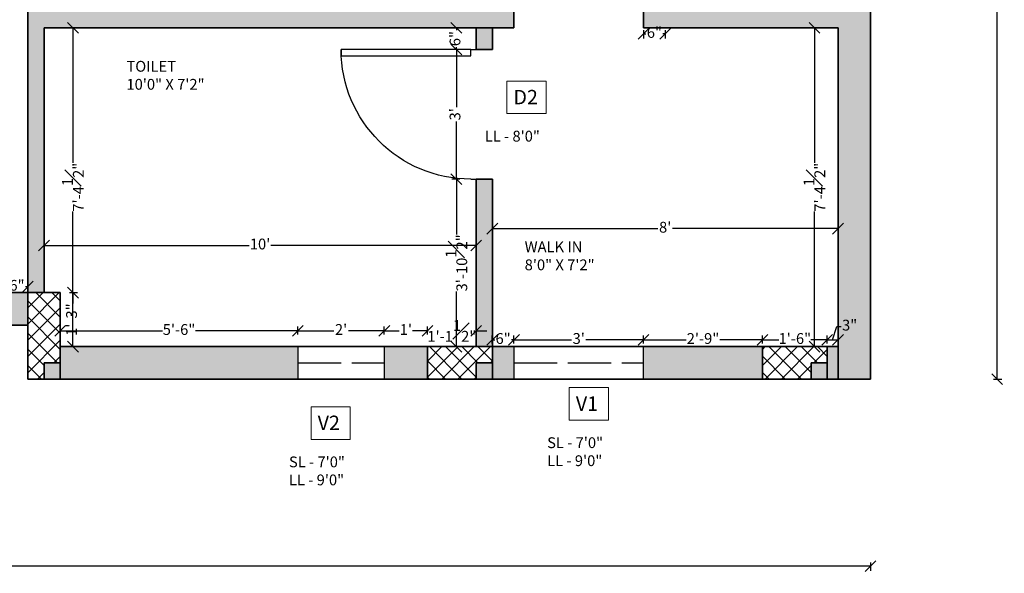
# Model space of a CAD drawing. Units: inches. Extents: x 1365 to 2091, y 1589 to 2091.
# Tile 6 of 8: x 1818 to 2091, y 1589 to 1743. Entities that reach past the tile are written whole.
import ezdxf

# ---------------------------------------------------------------- set-up
doc = ezdxf.new("R2010")
doc.units = ezdxf.units.IN
doc.linetypes.add('ACAD_ISO02W100', pattern=[15, 12, -3])
for name, color, linetype, lineweight in [('A-ANNO-DIMS', 2, 'Continuous', 18), ('A-ANNO-SYMB', 12, 'Continuous', 18), ('A-AREA-IDEN', 7, 'Continuous', 18), ('A-COLS', 7, 'Continuous', 35), ('A-COLS-MARK-PATT', 114, 'Continuous', 13), ('A-COLS-PATT', 1, 'Continuous', 13), ('A-DOOR', 4, 'Continuous', 25), ('A-GLAZ', 150, 'Continuous', 30), ('A-GLAZ-HIDN', 150, 'ACAD_ISO02W100', 30), ('A-WALL', 7, 'Continuous', 35), ('A-WALL-PATT', 253, 'Continuous', 13)]:
    doc.layers.add(name, color=color, linetype=linetype, lineweight=lineweight)
doc.styles.get("Standard").update_dxf_attribs({"font": 'arial.ttf'})
doc.dimstyles.new('ISO-25', dxfattribs={"dimtxt": 3, "dimasz": 3, "dimexe": 1.25, "dimexo": 0.625, "dimtad": 0, "dimlunit": 4, "dimtxsty": 'Standard', "dimblk": 'OBLIQUE', "dimcen": 2.5, "dimclrd": 254, "dimclre": 254, "dimclrt": 1, "dimadec": 0, "dimazin": 0, "dimtfac": 1, "dimtmove": 0, "dimatfit": 3, "dimfxl": 1, "dimfxlon": 1, "dimfrac": 1, "dimarcsym": 0})

# ---------------------------------------------------------------- blocks, each defined once
blk = doc.blocks.new('*U7')
for p, q in [((0, 0), (0, -6)), ((36, 0), (36, -6))]:
    blk.add_line(p, q)
blk.add_lwpolyline([(0, 0), (0, 36), (1.75, 36), (1.75, 0)], close=True)
blk.add_arc((0, 0), 36, 0, 90)
blk = doc.blocks.new('_Oblique')
at = {"color": 0, "linetype": 'ByBlock', "lineweight": -2}
blk.add_line((-0.5, -0.5), (0.5, 0.5), dxfattribs=at)
blk = doc.blocks.new('*D53')
at = {"layer": 'A-ANNO-DIMS', "color": 0, "lineweight": -2, "transparency": 16777216}
for p, q in [((1813.75, 1667.5), (1813.75, 1669.75)), ((1813.75, 1668.5), (1814.4, 1668.5)), ((1819.75, 1668.5), (1819.11, 1668.5)), ((1819.75, 1667.5), (1819.75, 1669.75))]:
    blk.add_line(p, q, dxfattribs=at)
at = {"layer": 'Defpoints', "color": 0, "transparency": 16777216}
for p in [(1819.75, 1668.5), (1813.75, 1666.86), (1819.75, 1666.86)]:
    blk.add_point(p, dxfattribs=at)
at = {"layer": 'A-ANNO-DIMS', "color": 0, "lineweight": -2, "transparency": 16777216, "xscale": 3, "yscale": 3, "zscale": 3, "rotation": 180}
blk.add_blockref('_Oblique', (1813.75, 1668.5), dxfattribs=at)
at = {"layer": 'A-ANNO-DIMS', "color": 0, "lineweight": -2, "transparency": 16777216, "xscale": 3, "yscale": 3, "zscale": 3}
blk.add_blockref('_Oblique', (1819.75, 1668.5), dxfattribs=at)
at = {"layer": 'A-ANNO-DIMS', "color": 0, "transparency": 16777216, "insert": (1816.75, 1668.5), "char_height": 3, "attachment_point": 5}
blk.add_mtext('6"', dxfattribs=at)
blk = doc.blocks.new('*D54')
at = {"layer": 'A-ANNO-DIMS', "color": 0, "lineweight": -2, "transparency": 16777216}
for p, q in [((1828.75, 1655.23), (1828.75, 1657.48)), ((1894.75, 1655.23), (1894.75, 1657.48)), ((1828.75, 1656.23), (1857.14, 1656.23)), ((1894.75, 1656.23), (1866.37, 1656.23))]:
    blk.add_line(p, q, dxfattribs=at)
at = {"layer": 'Defpoints', "color": 0, "transparency": 16777216}
for p in [(1894.75, 1656.23), (1828.75, 1651.86), (1894.75, 1651.86)]:
    blk.add_point(p, dxfattribs=at)
at = {"layer": 'A-ANNO-DIMS', "color": 0, "lineweight": -2, "transparency": 16777216, "xscale": 3, "yscale": 3, "zscale": 3, "rotation": 180}
blk.add_blockref('_Oblique', (1828.75, 1656.23), dxfattribs=at)
at = {"layer": 'A-ANNO-DIMS', "color": 0, "lineweight": -2, "transparency": 16777216, "xscale": 3, "yscale": 3, "zscale": 3}
blk.add_blockref('_Oblique', (1894.75, 1656.23), dxfattribs=at)
at = {"layer": 'A-ANNO-DIMS', "color": 0, "transparency": 16777216, "insert": (1861.75, 1656.23), "char_height": 3, "attachment_point": 5}
blk.add_mtext('5\'-6"', dxfattribs=at)
blk = doc.blocks.new('*D55')
at = {"layer": 'A-ANNO-DIMS', "color": 0, "lineweight": -2, "transparency": 16777216}
for p, q in [((1894.75, 1655.23), (1894.75, 1657.48)), ((1918.75, 1655.23), (1918.75, 1657.48)), ((1894.75, 1656.23), (1904.72, 1656.23)), ((1918.75, 1656.23), (1908.78, 1656.23))]:
    blk.add_line(p, q, dxfattribs=at)
at = {"layer": 'Defpoints', "color": 0, "transparency": 16777216}
for p in [(1918.75, 1656.23), (1894.75, 1651.86), (1918.75, 1651.86)]:
    blk.add_point(p, dxfattribs=at)
at = {"layer": 'A-ANNO-DIMS', "color": 0, "lineweight": -2, "transparency": 16777216, "xscale": 3, "yscale": 3, "zscale": 3, "rotation": 180}
blk.add_blockref('_Oblique', (1894.75, 1656.23), dxfattribs=at)
at = {"layer": 'A-ANNO-DIMS', "color": 0, "lineweight": -2, "transparency": 16777216, "xscale": 3, "yscale": 3, "zscale": 3}
blk.add_blockref('_Oblique', (1918.75, 1656.23), dxfattribs=at)
at = {"layer": 'A-ANNO-DIMS', "color": 0, "transparency": 16777216, "insert": (1906.75, 1656.23), "char_height": 3, "attachment_point": 5}
blk.add_mtext("2'", dxfattribs=at)
blk = doc.blocks.new('*D56')
at = {"layer": 'A-ANNO-DIMS', "color": 0, "lineweight": -2, "transparency": 16777216}
for p, q in [((1918.75, 1655.23), (1918.75, 1657.48)), ((1930.75, 1655.23), (1930.75, 1657.48)), ((1918.75, 1656.23), (1922.89, 1656.23)), ((1930.75, 1656.23), (1926.62, 1656.23))]:
    blk.add_line(p, q, dxfattribs=at)
at = {"layer": 'Defpoints', "color": 0, "transparency": 16777216}
for p in [(1930.75, 1656.23), (1918.75, 1651.86), (1930.75, 1651.86)]:
    blk.add_point(p, dxfattribs=at)
at = {"layer": 'A-ANNO-DIMS', "color": 0, "lineweight": -2, "transparency": 16777216, "xscale": 3, "yscale": 3, "zscale": 3, "rotation": 180}
blk.add_blockref('_Oblique', (1918.75, 1656.23), dxfattribs=at)
at = {"layer": 'A-ANNO-DIMS', "color": 0, "lineweight": -2, "transparency": 16777216, "xscale": 3, "yscale": 3, "zscale": 3}
blk.add_blockref('_Oblique', (1930.75, 1656.23), dxfattribs=at)
at = {"layer": 'A-ANNO-DIMS', "color": 0, "transparency": 16777216, "insert": (1924.75, 1656.23), "char_height": 3, "attachment_point": 5}
blk.add_mtext("1'", dxfattribs=at)
blk = doc.blocks.new('*D57')
at = {"layer": 'A-ANNO-DIMS', "color": 0, "lineweight": -2, "transparency": 16777216}
for p, q in [((1930.75, 1655.23), (1930.75, 1657.48)), ((1944.25, 1655.23), (1944.25, 1657.48)), ((1930.75, 1656.23), (1927.75, 1656.23)), ((1930.75, 1656.23), (1930.89, 1656.23)), ((1944.25, 1656.23), (1944.12, 1656.23)), ((1944.25, 1656.23), (1947.25, 1656.23))]:
    blk.add_line(p, q, dxfattribs=at)
at = {"layer": 'Defpoints', "color": 0, "transparency": 16777216}
for p in [(1944.25, 1656.23), (1930.75, 1651.86), (1944.25, 1651.86)]:
    blk.add_point(p, dxfattribs=at)
at = {"layer": 'A-ANNO-DIMS', "color": 0, "lineweight": -2, "transparency": 16777216, "xscale": 3, "yscale": 3, "zscale": 3}
blk.add_blockref('_Oblique', (1930.75, 1656.23), dxfattribs=at)
at = {"layer": 'A-ANNO-DIMS', "color": 0, "lineweight": -2, "transparency": 16777216, "xscale": 3, "yscale": 3, "zscale": 3, "rotation": 180}
blk.add_blockref('_Oblique', (1944.25, 1656.23), dxfattribs=at)
at = {"layer": 'A-ANNO-DIMS', "color": 0, "transparency": 16777216, "insert": (1937.5, 1656.23), "char_height": 3, "attachment_point": 5}
blk.add_mtext('1\'-1{\\H1x;\\S1#2;}"', dxfattribs=at)
blk = doc.blocks.new('*D58')
at = {"layer": 'A-ANNO-DIMS', "color": 0, "lineweight": -2, "transparency": 16777216}
for p, q in [((1831.29, 1666.86), (1833.54, 1666.86)), ((1832.29, 1666.86), (1832.29, 1663.83)), ((1832.29, 1651.86), (1832.29, 1654.89)), ((1831.29, 1651.86), (1833.54, 1651.86))]:
    blk.add_line(p, q, dxfattribs=at)
at = {"layer": 'Defpoints', "color": 0, "transparency": 16777216}
for p in [(1828.75, 1666.86), (1828.75, 1651.86), (1832.29, 1651.86)]:
    blk.add_point(p, dxfattribs=at)
at = {"layer": 'A-ANNO-DIMS', "color": 0, "lineweight": -2, "transparency": 16777216, "xscale": 3, "yscale": 3, "zscale": 3}
for p, rotation in [((1832.29, 1666.86), 90), ((1832.29, 1651.86), 270)]:
    blk.add_blockref('_Oblique', p, dxfattribs=dict(at, rotation=rotation))
at = {"layer": 'A-ANNO-DIMS', "color": 0, "transparency": 16777216, "insert": (1832.29, 1659.36), "char_height": 3, "attachment_point": 5, "rotation": 90}
blk.add_mtext('1\'-3"', dxfattribs=at)
blk = doc.blocks.new('*D59')
at = {"layer": 'A-ANNO-DIMS', "color": 0, "lineweight": -2, "transparency": 16777216}
for p, q in [((1832.29, 1740.36), (1833.54, 1740.36)), ((1832.29, 1740.36), (1832.29, 1702.85)), ((1832.29, 1651.86), (1832.29, 1689.36)), ((1831.29, 1651.86), (1833.54, 1651.86))]:
    blk.add_line(p, q, dxfattribs=at)
at = {"layer": 'Defpoints', "color": 0, "transparency": 16777216}
for p in [(1832.29, 1740.36), (1832.29, 1740.36), (1828.75, 1651.86)]:
    blk.add_point(p, dxfattribs=at)
at = {"layer": 'A-ANNO-DIMS', "color": 0, "lineweight": -2, "transparency": 16777216, "xscale": 3, "yscale": 3, "zscale": 3}
for p, rotation in [((1832.29, 1740.36), 90), ((1832.29, 1651.86), 270)]:
    blk.add_blockref('_Oblique', p, dxfattribs=dict(at, rotation=rotation))
at = {"layer": 'A-ANNO-DIMS', "color": 0, "transparency": 16777216, "insert": (1832.29, 1696.11), "char_height": 3, "attachment_point": 5, "rotation": 90}
blk.add_mtext('7\'-4{\\H1x;\\S1#2;}"', dxfattribs=at)
blk = doc.blocks.new('*D60')
at = {"layer": 'A-ANNO-DIMS', "color": 0, "lineweight": -2, "transparency": 16777216}
for p, q in [((1824.25, 1679.96), (1824.25, 1678.71)), ((1824.25, 1679.96), (1881.22, 1679.96)), ((1944.25, 1679.96), (1887.28, 1679.96)), ((1944.25, 1679.96), (1944.25, 1678.71))]:
    blk.add_line(p, q, dxfattribs=at)
at = {"layer": 'Defpoints', "color": 0, "transparency": 16777216}
for p in [(1824.25, 1680.4), (1944.25, 1680.4), (1944.25, 1679.96)]:
    blk.add_point(p, dxfattribs=at)
at = {"layer": 'A-ANNO-DIMS', "color": 0, "lineweight": -2, "transparency": 16777216, "xscale": 3, "yscale": 3, "zscale": 3, "rotation": 180}
blk.add_blockref('_Oblique', (1824.25, 1679.96), dxfattribs=at)
at = {"layer": 'A-ANNO-DIMS', "color": 0, "lineweight": -2, "transparency": 16777216, "xscale": 3, "yscale": 3, "zscale": 3}
blk.add_blockref('_Oblique', (1944.25, 1679.96), dxfattribs=at)
at = {"layer": 'A-ANNO-DIMS', "color": 0, "transparency": 16777216, "insert": (1884.25, 1679.96), "char_height": 3, "attachment_point": 5}
blk.add_mtext("10'", dxfattribs=at)
blk = doc.blocks.new('*D68')
at = {"layer": 'A-ANNO-DIMS', "color": 0, "lineweight": -2, "transparency": 16777216}
for p, q in [((1990.75, 1739.68), (1990.75, 1737.43)), ((1996.75, 1739.68), (1996.75, 1737.43)), ((1990.75, 1738.68), (1991.4, 1738.68)), ((1996.75, 1738.68), (1996.11, 1738.68))]:
    blk.add_line(p, q, dxfattribs=at)
at = {"layer": 'Defpoints', "color": 0, "transparency": 16777216}
for p in [(1990.75, 1744.86), (1996.75, 1744.86), (1996.75, 1738.68)]:
    blk.add_point(p, dxfattribs=at)
at = {"layer": 'A-ANNO-DIMS', "color": 0, "lineweight": -2, "transparency": 16777216, "xscale": 3, "yscale": 3, "zscale": 3, "rotation": 180}
blk.add_blockref('_Oblique', (1990.75, 1738.68), dxfattribs=at)
at = {"layer": 'A-ANNO-DIMS', "color": 0, "lineweight": -2, "transparency": 16777216, "xscale": 3, "yscale": 3, "zscale": 3}
blk.add_blockref('_Oblique', (1996.75, 1738.68), dxfattribs=at)
at = {"layer": 'A-ANNO-DIMS', "color": 0, "transparency": 16777216, "insert": (1993.75, 1738.68), "char_height": 3, "attachment_point": 5}
blk.add_mtext('6"', dxfattribs=at)
blk = doc.blocks.new('*D76')
at = {"layer": 'A-ANNO-DIMS', "color": 0, "lineweight": -2, "transparency": 16777216}
for p, q in [((1948.75, 1685.61), (1948.75, 1683.36)), ((1948.75, 1684.61), (1994.75, 1684.61)), ((2044.75, 1684.61), (1998.76, 1684.61)), ((2044.75, 1685.61), (2044.75, 1683.36))]:
    blk.add_line(p, q, dxfattribs=at)
at = {"layer": 'Defpoints', "color": 0, "transparency": 16777216}
for p in [(1948.75, 1686.34), (1948.75, 1684.61), (2044.75, 1686.34)]:
    blk.add_point(p, dxfattribs=at)
at = {"layer": 'A-ANNO-DIMS', "color": 0, "lineweight": -2, "transparency": 16777216, "xscale": 3, "yscale": 3, "zscale": 3, "rotation": 180}
blk.add_blockref('_Oblique', (1948.75, 1684.61), dxfattribs=at)
at = {"layer": 'A-ANNO-DIMS', "color": 0, "lineweight": -2, "transparency": 16777216, "xscale": 3, "yscale": 3, "zscale": 3}
blk.add_blockref('_Oblique', (2044.75, 1684.61), dxfattribs=at)
at = {"layer": 'A-ANNO-DIMS', "color": 0, "transparency": 16777216, "insert": (1996.75, 1684.61), "char_height": 3, "attachment_point": 5}
blk.add_mtext("8'", dxfattribs=at)
blk = doc.blocks.new('*D77')
at = {"layer": 'A-ANNO-DIMS', "color": 0, "lineweight": -2, "transparency": 16777216}
for p, q in [((2039.19, 1740.36), (2036.94, 1740.36)), ((2038.19, 1740.36), (2038.19, 1702.85)), ((2038.19, 1651.86), (2038.19, 1689.36)), ((2039.19, 1651.86), (2036.94, 1651.86))]:
    blk.add_line(p, q, dxfattribs=at)
at = {"layer": 'Defpoints', "color": 0, "transparency": 16777216}
for p in [(2044.75, 1740.36), (2038.19, 1651.86), (2044.75, 1651.86)]:
    blk.add_point(p, dxfattribs=at)
at = {"layer": 'A-ANNO-DIMS', "color": 0, "lineweight": -2, "transparency": 16777216, "xscale": 3, "yscale": 3, "zscale": 3}
for p, rotation in [((2038.19, 1740.36), 90), ((2038.19, 1651.86), 270)]:
    blk.add_blockref('_Oblique', p, dxfattribs=dict(at, rotation=rotation))
at = {"layer": 'A-ANNO-DIMS', "color": 0, "transparency": 16777216, "insert": (2038.19, 1696.11), "char_height": 3, "attachment_point": 5, "rotation": 90}
blk.add_mtext('7\'-4{\\H1x;\\S1#2;}"', dxfattribs=at)
blk = doc.blocks.new('*D78')
at = {"layer": 'A-ANNO-DIMS', "color": 0, "lineweight": -2, "transparency": 16777216}
for p, q in [((1948.75, 1652.73), (1948.75, 1654.98)), ((1954.75, 1652.73), (1954.75, 1654.98)), ((1948.75, 1653.73), (1949.4, 1653.73)), ((1954.75, 1653.73), (1954.11, 1653.73))]:
    blk.add_line(p, q, dxfattribs=at)
at = {"layer": 'Defpoints', "color": 0, "transparency": 16777216}
for p in [(1948.75, 1651.86), (1954.75, 1653.73), (1954.75, 1651.86)]:
    blk.add_point(p, dxfattribs=at)
at = {"layer": 'A-ANNO-DIMS', "color": 0, "lineweight": -2, "transparency": 16777216, "xscale": 3, "yscale": 3, "zscale": 3, "rotation": 180}
blk.add_blockref('_Oblique', (1948.75, 1653.73), dxfattribs=at)
at = {"layer": 'A-ANNO-DIMS', "color": 0, "lineweight": -2, "transparency": 16777216, "xscale": 3, "yscale": 3, "zscale": 3}
blk.add_blockref('_Oblique', (1954.75, 1653.73), dxfattribs=at)
at = {"layer": 'A-ANNO-DIMS', "color": 0, "transparency": 16777216, "insert": (1951.75, 1653.73), "char_height": 3, "attachment_point": 5}
blk.add_mtext('6"', dxfattribs=at)
blk = doc.blocks.new('*D79')
at = {"layer": 'A-ANNO-DIMS', "color": 0, "lineweight": -2, "transparency": 16777216}
for p, q in [((1954.75, 1652.73), (1954.75, 1654.98)), ((1990.75, 1652.73), (1990.75, 1654.98)), ((1954.75, 1653.73), (1970.75, 1653.73)), ((1990.75, 1653.73), (1974.76, 1653.73))]:
    blk.add_line(p, q, dxfattribs=at)
at = {"layer": 'Defpoints', "color": 0, "transparency": 16777216}
for p in [(1954.75, 1651.86), (1990.75, 1653.73), (1990.75, 1651.86)]:
    blk.add_point(p, dxfattribs=at)
at = {"layer": 'A-ANNO-DIMS', "color": 0, "lineweight": -2, "transparency": 16777216, "xscale": 3, "yscale": 3, "zscale": 3, "rotation": 180}
blk.add_blockref('_Oblique', (1954.75, 1653.73), dxfattribs=at)
at = {"layer": 'A-ANNO-DIMS', "color": 0, "lineweight": -2, "transparency": 16777216, "xscale": 3, "yscale": 3, "zscale": 3}
blk.add_blockref('_Oblique', (1990.75, 1653.73), dxfattribs=at)
at = {"layer": 'A-ANNO-DIMS', "color": 0, "transparency": 16777216, "insert": (1972.75, 1653.73), "char_height": 3, "attachment_point": 5}
blk.add_mtext("3'", dxfattribs=at)
blk = doc.blocks.new('*D80')
at = {"layer": 'A-ANNO-DIMS', "color": 0, "lineweight": -2, "transparency": 16777216}
for p, q in [((1990.75, 1652.73), (1990.75, 1654.98)), ((2023.75, 1652.73), (2023.75, 1654.98)), ((1990.75, 1653.73), (2002.62, 1653.73)), ((2023.75, 1653.73), (2011.89, 1653.73))]:
    blk.add_line(p, q, dxfattribs=at)
at = {"layer": 'Defpoints', "color": 0, "transparency": 16777216}
for p in [(1990.75, 1651.86), (2023.75, 1653.73), (2023.75, 1651.86)]:
    blk.add_point(p, dxfattribs=at)
at = {"layer": 'A-ANNO-DIMS', "color": 0, "lineweight": -2, "transparency": 16777216, "xscale": 3, "yscale": 3, "zscale": 3, "rotation": 180}
blk.add_blockref('_Oblique', (1990.75, 1653.73), dxfattribs=at)
at = {"layer": 'A-ANNO-DIMS', "color": 0, "lineweight": -2, "transparency": 16777216, "xscale": 3, "yscale": 3, "zscale": 3}
blk.add_blockref('_Oblique', (2023.75, 1653.73), dxfattribs=at)
at = {"layer": 'A-ANNO-DIMS', "color": 0, "transparency": 16777216, "insert": (2007.25, 1653.73), "char_height": 3, "attachment_point": 5}
blk.add_mtext('2\'-9"', dxfattribs=at)
blk = doc.blocks.new('*D81')
at = {"layer": 'A-ANNO-DIMS', "color": 0, "lineweight": -2, "transparency": 16777216}
for p, q in [((2023.75, 1652.73), (2023.75, 1654.98)), ((2041.75, 1652.73), (2041.75, 1654.98)), ((2023.75, 1653.73), (2028.28, 1653.73)), ((2041.75, 1653.73), (2037.22, 1653.73))]:
    blk.add_line(p, q, dxfattribs=at)
at = {"layer": 'Defpoints', "color": 0, "transparency": 16777216}
for p in [(2023.75, 1651.86), (2041.75, 1653.73), (2041.75, 1651.86)]:
    blk.add_point(p, dxfattribs=at)
at = {"layer": 'A-ANNO-DIMS', "color": 0, "lineweight": -2, "transparency": 16777216, "xscale": 3, "yscale": 3, "zscale": 3, "rotation": 180}
blk.add_blockref('_Oblique', (2023.75, 1653.73), dxfattribs=at)
at = {"layer": 'A-ANNO-DIMS', "color": 0, "lineweight": -2, "transparency": 16777216, "xscale": 3, "yscale": 3, "zscale": 3}
blk.add_blockref('_Oblique', (2041.75, 1653.73), dxfattribs=at)
at = {"layer": 'A-ANNO-DIMS', "color": 0, "transparency": 16777216, "insert": (2032.75, 1653.73), "char_height": 3, "attachment_point": 5}
blk.add_mtext('1\'-6"', dxfattribs=at)
blk = doc.blocks.new('*D82')
at = {"layer": 'A-ANNO-DIMS', "color": 0, "lineweight": -2, "transparency": 16777216}
for p, q in [((2043.25, 1653.73), (2044.37, 1657.45)), ((2044.37, 1657.45), (2045.62, 1657.45)), ((2041.75, 1652.73), (2041.75, 1654.98)), ((2044.75, 1652.73), (2044.75, 1654.98)), ((2041.75, 1653.73), (2044.75, 1653.73))]:
    blk.add_line(p, q, dxfattribs=at)
at = {"layer": 'Defpoints', "color": 0, "transparency": 16777216}
for p in [(2041.75, 1651.86), (2044.75, 1653.73), (2044.75, 1651.86)]:
    blk.add_point(p, dxfattribs=at)
at = {"layer": 'A-ANNO-DIMS', "color": 0, "lineweight": -2, "transparency": 16777216, "xscale": 3, "yscale": 3, "zscale": 3, "rotation": 180}
blk.add_blockref('_Oblique', (2041.75, 1653.73), dxfattribs=at)
at = {"layer": 'A-ANNO-DIMS', "color": 0, "lineweight": -2, "transparency": 16777216, "xscale": 3, "yscale": 3, "zscale": 3}
blk.add_blockref('_Oblique', (2044.75, 1653.73), dxfattribs=at)
at = {"layer": 'A-ANNO-DIMS', "color": 0, "transparency": 16777216, "insert": (2047.97, 1657.45), "char_height": 3, "attachment_point": 5}
blk.add_mtext('3"', dxfattribs=at)
blk = doc.blocks.new('*D83')
at = {"layer": 'A-ANNO-DIMS', "color": 0, "lineweight": -2, "transparency": 16777216}
for p, q in [((1939.77, 1740.36), (1937.52, 1740.36)), ((1938.77, 1740.36), (1938.77, 1739.71)), ((1939.77, 1734.36), (1937.52, 1734.36)), ((1938.77, 1734.36), (1938.77, 1735))]:
    blk.add_line(p, q, dxfattribs=at)
at = {"layer": 'Defpoints', "color": 0, "transparency": 16777216}
for p in [(1944.25, 1740.36), (1938.77, 1734.36), (1944.25, 1734.36)]:
    blk.add_point(p, dxfattribs=at)
at = {"layer": 'A-ANNO-DIMS', "color": 0, "lineweight": -2, "transparency": 16777216, "xscale": 3, "yscale": 3, "zscale": 3}
for p, rotation in [((1938.77, 1740.36), 90), ((1938.77, 1734.36), 270)]:
    blk.add_blockref('_Oblique', p, dxfattribs=dict(at, rotation=rotation))
at = {"layer": 'A-ANNO-DIMS', "color": 0, "transparency": 16777216, "insert": (1938.77, 1737.36), "char_height": 3, "attachment_point": 5, "rotation": 90}
blk.add_mtext('6"', dxfattribs=at)
blk = doc.blocks.new('*D84')
at = {"layer": 'A-ANNO-DIMS', "color": 0, "lineweight": -2, "transparency": 16777216}
for p, q in [((1939.77, 1734.36), (1937.52, 1734.36)), ((1938.77, 1734.36), (1938.77, 1718.36)), ((1938.77, 1698.36), (1938.77, 1714.35)), ((1939.77, 1698.36), (1937.52, 1698.36))]:
    blk.add_line(p, q, dxfattribs=at)
at = {"layer": 'Defpoints', "color": 0, "transparency": 16777216}
for p in [(1944.25, 1734.36), (1938.77, 1698.36), (1944.25, 1698.36)]:
    blk.add_point(p, dxfattribs=at)
at = {"layer": 'A-ANNO-DIMS', "color": 0, "lineweight": -2, "transparency": 16777216, "xscale": 3, "yscale": 3, "zscale": 3}
for p, rotation in [((1938.77, 1734.36), 90), ((1938.77, 1698.36), 270)]:
    blk.add_blockref('_Oblique', p, dxfattribs=dict(at, rotation=rotation))
at = {"layer": 'A-ANNO-DIMS', "color": 0, "transparency": 16777216, "insert": (1938.77, 1716.36), "char_height": 3, "attachment_point": 5, "rotation": 90}
blk.add_mtext("3'", dxfattribs=at)
blk = doc.blocks.new('*D85')
at = {"layer": 'A-ANNO-DIMS', "color": 0, "lineweight": -2, "transparency": 16777216}
for p, q in [((1939.77, 1698.36), (1937.52, 1698.36)), ((1938.77, 1698.36), (1938.77, 1683.03)), ((1938.77, 1651.86), (1938.77, 1667.18)), ((1939.77, 1651.86), (1937.52, 1651.86))]:
    blk.add_line(p, q, dxfattribs=at)
at = {"layer": 'Defpoints', "color": 0, "transparency": 16777216}
for p in [(1944.25, 1698.36), (1938.77, 1651.86), (1944.25, 1651.86)]:
    blk.add_point(p, dxfattribs=at)
at = {"layer": 'A-ANNO-DIMS', "color": 0, "lineweight": -2, "transparency": 16777216, "xscale": 3, "yscale": 3, "zscale": 3}
for p, rotation in [((1938.77, 1698.36), 90), ((1938.77, 1651.86), 270)]:
    blk.add_blockref('_Oblique', p, dxfattribs=dict(at, rotation=rotation))
at = {"layer": 'A-ANNO-DIMS', "color": 0, "transparency": 16777216, "insert": (1938.77, 1675.11), "char_height": 3, "attachment_point": 5, "rotation": 90}
blk.add_mtext('3\'-10{\\H1x;\\S1#2;}"', dxfattribs=at)
blk = doc.blocks.new('OPENING-TAG-V2')
blk.add_lwpolyline([(6.13, 13.79), (17.02, 13.79), (17.02, 4.75), (6.13, 4.75)], close=True)
at = {"attachment_point": 1}
for s, width, insert, char_height in [('{V2}', 14.5136, (7.98, 11.34), 4), ('{SL - 7\'0"\\PLL - 9\'0"}', 24.3857, (0, 0), 3)]:
    blk.add_mtext_dynamic_manual_height_columns(s, width=width, gutter_width=12.5, heights=[0], dxfattribs=dict(at, insert=insert, char_height=char_height))
blk = doc.blocks.new('OPENING-TAG-D2')
blk.add_lwpolyline([(6.13, 13.79), (17.02, 13.79), (17.02, 4.75), (6.13, 4.75)], close=True)
at = {"attachment_point": 1}
for s, width, insert, char_height in [('{D2}', 14.5136, (7.98, 11.34), 4), ('{LL - 8\'0"}', 24.3857, (0, 0), 3)]:
    blk.add_mtext_dynamic_manual_height_columns(s, width=width, gutter_width=12.5, heights=[0], dxfattribs=dict(at, insert=insert, char_height=char_height))
blk = doc.blocks.new('*D122')
at = {"layer": 'A-ANNO-DIMS', "color": 254, "lineweight": -2, "transparency": 16777216}
for p, q in [((1393.75, 1591.92), (1393.75, 1589.67)), ((2053.75, 1591.92), (2053.75, 1589.67)), ((1393.75, 1590.92), (1717.98, 1590.92)), ((2053.75, 1590.92), (1729.53, 1590.92))]:
    blk.add_line(p, q, dxfattribs=at)
at = {"layer": 'Defpoints', "color": 0, "transparency": 16777216}
for p in [(1393.75, 1642.86), (2053.75, 1642.86), (2053.75, 1590.92)]:
    blk.add_point(p, dxfattribs=at)
at = {"layer": 'A-ANNO-DIMS', "color": 254, "lineweight": -2, "transparency": 16777216, "xscale": 3, "yscale": 3, "zscale": 3, "rotation": 180}
blk.add_blockref('_Oblique', (1393.75, 1590.92), dxfattribs=at)
at = {"layer": 'A-ANNO-DIMS', "color": 254, "lineweight": -2, "transparency": 16777216, "xscale": 3, "yscale": 3, "zscale": 3}
blk.add_blockref('_Oblique', (2053.75, 1590.92), dxfattribs=at)
at = {"layer": 'A-ANNO-DIMS', "color": 1, "transparency": 16777216, "insert": (1723.75, 1590.92), "char_height": 3, "attachment_point": 5}
blk.add_mtext('55\'-0"', dxfattribs=at)
blk = doc.blocks.new('*D123')
at = {"layer": 'A-ANNO-DIMS', "color": 254, "lineweight": -2, "transparency": 16777216}
for p, q in [((2087.95, 2062.86), (2090.2, 2062.86)), ((2088.95, 2062.86), (2088.95, 1858.63)), ((2088.95, 1642.86), (2088.95, 1847.08)), ((2087.95, 1642.86), (2090.2, 1642.86))]:
    blk.add_line(p, q, dxfattribs=at)
at = {"layer": 'Defpoints', "color": 0, "transparency": 16777216}
for p in [(2053.75, 2062.86), (2088.95, 2062.86), (2053.75, 1642.86)]:
    blk.add_point(p, dxfattribs=at)
at = {"layer": 'A-ANNO-DIMS', "color": 254, "lineweight": -2, "transparency": 16777216, "xscale": 3, "yscale": 3, "zscale": 3}
for p, rotation in [((2088.95, 2062.86), 90), ((2088.95, 1642.86), 270)]:
    blk.add_blockref('_Oblique', p, dxfattribs=dict(at, rotation=rotation))
at = {"layer": 'A-ANNO-DIMS', "color": 1, "transparency": 16777216, "insert": (2088.95, 1852.86), "char_height": 3, "attachment_point": 5, "rotation": 90}
blk.add_mtext('35\'-0"', dxfattribs=at)

msp = doc.modelspace()

# ---------------------------------------------------------------- hatches: boundary and pattern name
at = {"layer": 'A-COLS-MARK-PATT'}
h = msp.add_hatch(color=256, dxfattribs=at)
h.dxf.hatch_style = 1
h.paths.add_polyline_path([(1398.254, 2062.858), (1393.754, 2062.858), (1393.754, 2058.358), (1398.254, 2058.358)])
h.paths.add_polyline_path([(1398.254, 1872.358), (1393.754, 1872.358), (1393.754, 1867.858), (1398.254, 1867.858)])
h.paths.add_polyline_path([(1398.254, 1807.858), (1393.754, 1807.858), (1393.754, 1803.358), (1398.254, 1803.358)])
h.paths.add_polyline_path([(1398.254, 1647.358), (1393.754, 1647.358), (1393.754, 1642.858), (1398.254, 1642.858)])
h.paths.add_polyline_path([(1638.254, 1647.358), (1633.754, 1647.358), (1633.754, 1642.858), (1638.254, 1642.858)])
h.paths.add_polyline_path([(1638.254, 1732.858), (1633.754, 1732.858), (1633.754, 1728.358), (1638.254, 1728.358)])
h.paths.add_polyline_path([(1647.254, 1876.858), (1642.754, 1876.858), (1642.754, 1872.358), (1647.254, 1872.358)])
h.paths.add_polyline_path([(1647.254, 1803.358), (1642.754, 1803.358), (1642.754, 1798.858), (1647.254, 1798.858)])
h.paths.add_polyline_path([(1647.254, 2062.858), (1642.754, 2062.858), (1642.754, 2058.358), (1647.254, 2058.358)])
h.paths.add_polyline_path([(1824.254, 2062.858), (1819.754, 2062.858), (1819.754, 2058.358), (1824.254, 2058.358)])
h.paths.add_polyline_path([(1824.254, 1885.858), (1819.754, 1885.858), (1819.754, 1881.358), (1824.254, 1881.358)])
h.paths.add_polyline_path([(1828.754, 1647.358), (1824.254, 1647.358), (1824.254, 1642.858), (1828.754, 1642.858)])
h.paths.add_polyline_path([(1948.754, 1647.358), (1944.254, 1647.358), (1944.254, 1642.858), (1948.754, 1642.858)])
h.paths.add_polyline_path([(2041.754, 1647.358), (2037.254, 1647.358), (2037.254, 1642.858), (2041.754, 1642.858)])
h.paths.add_polyline_path([(2041.754, 1885.858), (2037.254, 1885.858), (2037.254, 1881.358), (2041.754, 1881.358)])
h.paths.add_polyline_path([(2041.754, 2062.858), (2037.254, 2062.858), (2037.254, 2058.358), (2041.754, 2058.358)])
at = {"layer": 'A-COLS-PATT'}
h = msp.add_hatch(dxfattribs=at)
h.set_pattern_fill('ANSI37', color=256)
h.paths.add_polyline_path([(1642.754, 1803.358), (1647.254, 1803.358), (1647.254, 1807.858), (1629.254, 1807.858), (1629.254, 1798.858), (1633.754, 1798.858), (1642.754, 1798.858)])
h.paths.add_polyline_path([(1647.254, 1872.358), (1642.754, 1872.358), (1642.754, 1876.858), (1641.254, 1876.858), (1623.254, 1876.858), (1623.254, 1867.858), (1638.254, 1867.858), (1647.254, 1867.858)])
h.paths.add_polyline_path([(1647.254, 2058.358), (1642.754, 2058.358), (1642.754, 2062.858), (1638.254, 2062.858), (1638.254, 2053.858), (1647.254, 2053.858)])
h.paths.add_polyline_path([(1642.754, 2053.858), (1638.254, 2053.858), (1638.254, 2041.858), (1642.754, 2041.858)])
h.paths.add_polyline_path([(1647.254, 2053.858), (1642.754, 2053.858), (1642.754, 2041.858), (1647.254, 2041.858)])
h.paths.add_polyline_path([(1828.754, 2062.858), (1824.254, 2062.858), (1824.254, 2058.358), (1819.754, 2058.358), (1819.754, 2038.858), (1828.754, 2038.858)])
h.paths.add_polyline_path([(1839.254, 1885.858), (1825.754, 1885.858), (1824.254, 1885.858), (1824.254, 1881.358), (1819.754, 1881.358), (1819.754, 1876.858), (1839.254, 1876.858)])
h.paths.add_polyline_path([(2041.754, 1881.358), (2037.254, 1881.358), (2037.254, 1885.858), (2023.754, 1885.858), (2023.754, 1876.858), (2041.754, 1876.858)])
h.paths.add_polyline_path([(1828.754, 1666.858), (1819.754, 1666.858), (1819.754, 1642.858), (1824.254, 1642.858), (1824.254, 1647.358), (1828.754, 1647.358)])
h.paths.add_polyline_path([(1944.254, 1647.358), (1948.754, 1647.358), (1948.754, 1651.858), (1930.754, 1651.858), (1930.754, 1642.858), (1944.254, 1642.858)])
h.paths.add_polyline_path([(2037.254, 1647.358), (2041.754, 1647.358), (2041.754, 1651.858), (2023.754, 1651.858), (2023.754, 1642.858), (2037.254, 1642.858)])
at = {"layer": 'A-WALL-PATT'}
h = msp.add_hatch(color=256, dxfattribs=at)
h.dxf.hatch_style = 1
h.paths.add_polyline_path([(1996.754, 1876.858), (1996.754, 1861.858), (2005.754, 1861.858), (2005.754, 1876.858), (2023.754, 1876.858), (2023.754, 1885.858), (1839.254, 1885.858), (1839.254, 1876.858)])
h.paths.add_polyline_path([(2053.754, 1744.858), (2005.754, 1744.858), (2005.754, 1765.858), (1996.754, 1765.858), (1996.754, 1744.858), (1990.754, 1744.858), (1990.754, 1740.358), (2044.754, 1740.358), (2044.754, 1651.858), (2044.754, 1642.858), (2053.754, 1642.858)])
h = msp.add_hatch(color=256, dxfattribs=at)
h.dxf.hatch_style = 1
h.paths.add_polyline_path([(1402.754, 1753.858), (1393.754, 1753.858), (1393.754, 1663.858), (1402.754, 1663.858)])
h.paths.add_polyline_path([(1533.254, 1804.358), (1476.254, 1804.358), (1476.254, 1816.358), (1471.754, 1816.358), (1471.754, 1804.358), (1402.754, 1804.358), (1402.754, 1799.858), (1533.254, 1799.858)])
h.paths.add_polyline_path([(1638.254, 1714.858), (1633.754, 1714.858), (1633.754, 1666.858), (1638.254, 1666.858)])
h.paths.add_polyline_path([(1638.254, 1740.858), (1633.754, 1740.858), (1633.754, 1732.858), (1638.254, 1732.858)])
h.paths.add_polyline_path([(1954.754, 1744.858), (1948.754, 1744.858), (1944.254, 1744.858), (1824.254, 1744.858), (1824.254, 1821.858), (1819.754, 1821.858), (1819.754, 1666.858), (1824.254, 1666.858), (1824.254, 1740.358), (1944.254, 1740.358), (1948.754, 1740.358), (1954.754, 1740.358)])
h.paths.add_polyline_path([(1948.754, 1698.358), (1944.254, 1698.358), (1944.254, 1651.858), (1948.754, 1651.858)])
h.paths.add_polyline_path([(1948.754, 1740.358), (1944.254, 1740.358), (1944.254, 1734.358), (1948.754, 1734.358)], flags=17)
h = msp.add_hatch(color=256, dxfattribs=at)
h.dxf.hatch_style = 1
h.paths.add_polyline_path([(1789.754, 1666.858), (1668.254, 1666.858), (1668.254, 1657.858), (1789.754, 1657.858)])
h.paths.add_polyline_path([(1644.254, 1666.858), (1638.254, 1666.858), (1638.254, 1657.858), (1644.254, 1657.858)])
h.paths.add_polyline_path([(1819.754, 1666.858), (1813.754, 1666.858), (1813.754, 1657.858), (1819.754, 1657.858)])
h = msp.add_hatch(color=256, dxfattribs=at)
h.dxf.hatch_style = 1
h.paths.add_polyline_path([(1894.754, 1651.858), (1828.754, 1651.858), (1828.754, 1642.858), (1894.754, 1642.858)])
h = msp.add_hatch(color=256, dxfattribs=at)
h.dxf.hatch_style = 1
h.paths.add_polyline_path([(1930.754, 1651.858), (1918.754, 1651.858), (1918.754, 1642.858), (1930.754, 1642.858)])
h.paths.add_polyline_path([(2044.754, 1651.858), (2041.754, 1651.858), (2041.754, 1642.858), (2044.754, 1642.858)])
h = msp.add_hatch(color=256, dxfattribs=at)
h.dxf.hatch_style = 1
h.paths.add_polyline_path([(1954.754, 1651.858), (1948.754, 1651.858), (1948.754, 1642.858), (1954.754, 1642.858)])
h = msp.add_hatch(color=256, dxfattribs=at)
h.dxf.hatch_style = 1
h.paths.add_polyline_path([(2023.754, 1651.858), (1990.754, 1651.858), (1990.754, 1642.858), (2023.754, 1642.858)])

# ---------------------------------------------------------------- linework, layer by layer
at = {"layer": 'A-ANNO-SYMB'}
msp.add_lwpolyline([(1970.101, 1640.491), (1980.99, 1640.491), (1980.99, 1631.453), (1970.101, 1631.453)], close=True, dxfattribs=at)
at = {"layer": 'A-COLS'}
for p, q in [((1819.754, 1666.858), (1828.754, 1666.858)), ((1828.754, 1666.858), (1828.754, 1642.858)), ((1930.754, 1642.858), (1930.754, 1651.858)), ((2023.754, 1651.858), (2023.754, 1642.858)), ((2041.754, 1651.858), (2041.754, 1642.858)), ((1824.254, 1642.858), (1824.254, 1647.358)), ((1824.254, 1647.358), (1828.754, 1647.358)), ((1944.254, 1642.858), (1944.254, 1647.358)), ((1944.254, 1647.358), (1948.754, 1647.358)), ((2041.754, 1647.358), (2037.254, 1647.358)), ((2037.254, 1647.358), (2037.254, 1642.858)), ((1828.754, 1642.858), (1824.254, 1642.858)), ((1944.254, 1642.858), (1930.754, 1642.858)), ((1948.754, 1642.858), (1944.254, 1642.858))]:
    msp.add_line(p, q, dxfattribs=at)
at = {"layer": 'A-GLAZ'}
for p, q in [((1894.754, 1651.858), (1894.754, 1642.858)), ((1918.754, 1651.858), (1918.754, 1642.858)), ((1954.754, 1651.858), (1954.754, 1642.858)), ((1990.754, 1642.858), (1990.754, 1651.858)), ((1954.754, 1642.858), (1990.754, 1642.858))]:
    msp.add_line(p, q, dxfattribs=at)
at = {"layer": 'A-GLAZ-HIDN'}
for p, q in [((1894.754, 1647.358), (1918.754, 1647.358)), ((1954.754, 1647.358), (1990.754, 1647.358))]:
    msp.add_line(p, q, dxfattribs=at)
at = {"layer": 'A-WALL'}
for p, q in [((2053.754, 1885.858), (2053.754, 1642.858)), ((1819.754, 1821.858), (1819.754, 1666.858)), ((1954.754, 1744.858), (1954.754, 1740.358)), ((1990.754, 1740.358), (1990.754, 1744.858)), ((1944.254, 1740.358), (1824.254, 1740.358)), ((1824.254, 1740.358), (1824.254, 1666.858)), ((1948.754, 1740.358), (1944.254, 1740.358)), ((1944.254, 1734.358), (1944.254, 1740.358)), ((1954.754, 1740.358), (1948.754, 1740.358)), ((1954.754, 1740.358), (1948.754, 1740.358)), ((1948.754, 1740.358), (1948.754, 1734.358)), ((2044.754, 1740.358), (1990.754, 1740.358)), ((2044.754, 1651.858), (2044.754, 1740.358)), ((1948.754, 1734.358), (1944.254, 1734.358)), ((1944.254, 1651.858), (1944.254, 1698.358)), ((1944.254, 1698.358), (1948.754, 1698.358)), ((1948.754, 1698.358), (1948.754, 1642.858)), ((1813.754, 1666.858), (1819.754, 1666.858)), ((1819.754, 1666.858), (1819.754, 1642.858)), ((1813.754, 1657.858), (1819.754, 1657.858)), ((1828.754, 1651.858), (2044.754, 1651.858)), ((1828.754, 1651.858), (1894.754, 1651.858)), ((2044.754, 1651.858), (2044.754, 1642.858)), ((1819.754, 1642.858), (2053.754, 1642.858))]:
    msp.add_line(p, q, dxfattribs=at)

# ---------------------------------------------------------------- block references
at = {"layer": 'A-ANNO-SYMB'}
for name, p in [('OPENING-TAG-D2', (1946.639, 1711.778)), ('OPENING-TAG-V2', (1892.273, 1621.372))]:
    msp.add_blockref(name, p, dxfattribs=at)
at = {"layer": 'A-DOOR', "xscale": -1, "rotation": 90}
msp.add_blockref('*U7', (1942.754, 1734.358), dxfattribs=at)

# ---------------------------------------------------------------- texts
at = {"layer": 'A-ANNO-SYMB', "attachment_point": 1}
for s, width, insert, char_height in [('{V1}', 14.51356, (1971.941, 1638.04), 4), ('{SL - 7\'0"\\PLL - 9\'0"}', 24.3857, (1963.966, 1626.704), 3)]:
    msp.add_mtext_dynamic_manual_height_columns(s, width=width, gutter_width=12.5, heights=[0], dxfattribs=dict(at, insert=insert, char_height=char_height))
at = {"layer": 'A-AREA-IDEN', "char_height": 3, "attachment_point": 1}
for s, insert in [('{TOILET\\P10\'0" X 7\'2"}', (1847.148, 1731.174)), ('{WALK IN\\P8\'0" X 7\'2"}', (1957.73, 1681.073))]:
    msp.add_mtext_dynamic_manual_height_columns(s, width=33.58604, gutter_width=12.5, heights=[0], dxfattribs=dict(at, insert=insert))

# ---------------------------------------------------------------- dimensions: what is measured, and where the dimension line sits
at = {"layer": 'A-ANNO-DIMS'}
for base, p1, p2, override, picture, middle in [((2088.954, 2062.858), (2053.754, 1642.858), (2053.754, 2062.858), {"dimdec": 1, "dimlfac": 1, "dimrnd": 0, "dimzin": 1, "dimdsep": 46, "dimlunit": 4, "dimfrac": 2}, '*D123', (2088.954, 1852.858)), ((1832.29, 1740.358), (1828.754, 1651.858), (1832.29, 1740.358), {"dimclrd": 0, "dimclre": 0, "dimclrt": 0, "dimtmove": 1}, '*D59', (1832.29, 1696.108)), ((1938.77, 1734.358), (1944.254, 1740.358), (1944.254, 1734.358), {"dimclrd": 0, "dimclre": 0, "dimclrt": 0}, '*D83', (1938.77, 1737.358)), ((2038.194, 1651.858), (2044.754, 1740.358), (2044.754, 1651.858), {"dimclrd": 0, "dimclre": 0, "dimclrt": 0}, '*D77', (2038.194, 1696.108)), ((1938.77, 1698.358), (1944.254, 1734.358), (1944.254, 1698.358), {"dimclrd": 0, "dimclre": 0, "dimclrt": 0, "dimtmove": 1}, '*D84', (1938.77, 1716.358)), ((1938.77, 1651.858), (1944.254, 1698.358), (1944.254, 1651.858), {"dimclrd": 0, "dimclre": 0, "dimclrt": 0, "dimtmove": 1}, '*D85', (1938.77, 1675.108)), ((1832.29, 1651.858), (1828.754, 1666.858), (1828.754, 1651.858), {"dimclrd": 0, "dimclre": 0, "dimclrt": 0}, '*D58', (1832.29, 1659.358))]:
    dim = msp.add_linear_dim(base=base, p1=p1, p2=p2, angle=90, dimstyle='ISO-25', override=override, dxfattribs=at)
    dim.commit()
    dim.dimension.update_dxf_attribs({"geometry": picture, "text_midpoint": middle})
for base, p1, p2, override, picture, middle in [((1996.754, 1738.678), (1990.754, 1744.858), (1996.754, 1744.858), {"dimclrd": 0, "dimclre": 0, "dimclrt": 0}, '*D68', (1993.754, 1738.678)), ((1948.754, 1684.607), (2044.754, 1686.337), (1948.754, 1686.337), {"dimclrd": 0, "dimclre": 0, "dimclrt": 0}, '*D76', (1996.754, 1684.607)), ((1944.254, 1679.963), (1824.254, 1680.402), (1944.254, 1680.402), {"dimclrd": 0, "dimclre": 0, "dimclrt": 0}, '*D60', (1884.254, 1679.963)), ((1819.754, 1668.5), (1813.754, 1666.858), (1819.754, 1666.858), {"dimclrd": 0, "dimclre": 0, "dimclrt": 0, "dimtmove": 1}, '*D53', (1816.754, 1668.5)), ((1894.754, 1656.234), (1828.754, 1651.858), (1894.754, 1651.858), {"dimclrd": 0, "dimclre": 0, "dimclrt": 0}, '*D54', (1861.754, 1656.234)), ((1918.754, 1656.234), (1894.754, 1651.858), (1918.754, 1651.858), {"dimclrd": 0, "dimclre": 0, "dimclrt": 0, "dimtmove": 1}, '*D55', (1906.754, 1656.234)), ((1930.754, 1656.234), (1918.754, 1651.858), (1930.754, 1651.858), {"dimclrd": 0, "dimclre": 0, "dimclrt": 0, "dimtmove": 1}, '*D56', (1924.754, 1656.234)), ((1944.254, 1656.234), (1930.754, 1651.858), (1944.254, 1651.858), {"dimclrd": 0, "dimclre": 0, "dimclrt": 0, "dimtmove": 1}, '*D57', (1937.504, 1656.234)), ((2044.754, 1653.729), (2041.754, 1651.858), (2044.754, 1651.858), {"dimclrd": 0, "dimclre": 0, "dimclrt": 0, "dimtmove": 1}, '*D82', (2046.245, 1657.449)), ((1954.754, 1653.729), (1948.754, 1651.858), (1954.754, 1651.858), {"dimclrd": 0, "dimclre": 0, "dimclrt": 0}, '*D78', (1951.754, 1653.729)), ((1990.754, 1653.729), (1954.754, 1651.858), (1990.754, 1651.858), {"dimclrd": 0, "dimclre": 0, "dimclrt": 0, "dimtmove": 1}, '*D79', (1972.754, 1653.729)), ((2023.754, 1653.729), (1990.754, 1651.858), (2023.754, 1651.858), {"dimclrd": 0, "dimclre": 0, "dimclrt": 0, "dimtmove": 1}, '*D80', (2007.254, 1653.729)), ((2041.754, 1653.729), (2023.754, 1651.858), (2041.754, 1651.858), {"dimclrd": 0, "dimclre": 0, "dimclrt": 0, "dimtmove": 1}, '*D81', (2032.754, 1653.729)), ((2053.754, 1590.921), (1393.754, 1642.858), (2053.754, 1642.858), {"dimdec": 1, "dimlfac": 1, "dimrnd": 0, "dimzin": 1, "dimdsep": 46, "dimlunit": 4, "dimfrac": 2}, '*D122', (1723.754, 1590.921))]:
    dim = msp.add_linear_dim(base=base, p1=p1, p2=p2, dimstyle='ISO-25', override=override, dxfattribs=at)
    dim.commit()
    dim.dimension.update_dxf_attribs({"geometry": picture, "text_midpoint": middle})

doc.saveas('drawing.dxf')
